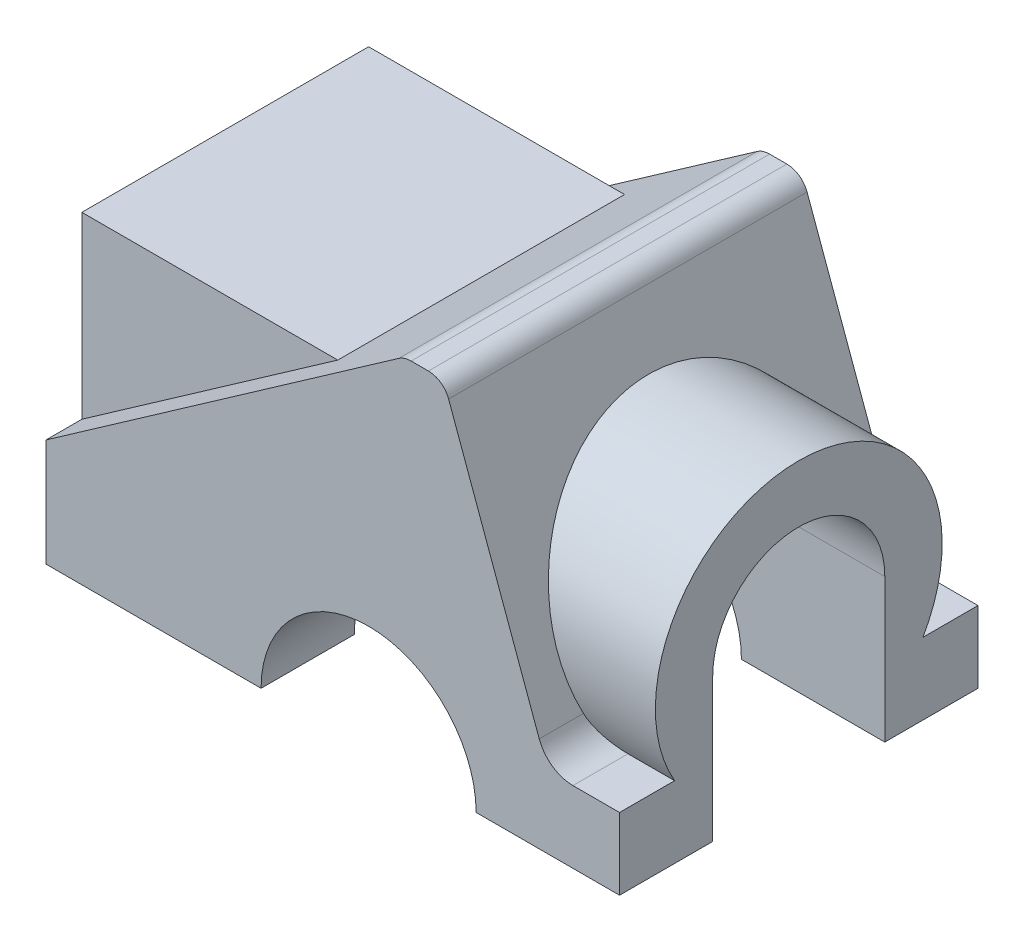
ISO-10303-21;
HEADER;
FILE_DESCRIPTION(('STEP AP214'),'2;1');
FILE_NAME('part.step','',(''),(''),'','','');
FILE_SCHEMA(('AUTOMOTIVE_DESIGN { 1 0 10303 214 1 1 1 1 }'));
ENDSEC;
DATA;
#1=APPLICATION_CONTEXT('core data for automotive mechanical design processes');
#2=APPLICATION_PROTOCOL_DEFINITION('international standard','automotive_design',2000,#1);
#3=PRODUCT_CONTEXT('',#1,'mechanical');
#4=PRODUCT('Part','Part','',(#3));
#5=PRODUCT_RELATED_PRODUCT_CATEGORY('part','',(#4));
#6=PRODUCT_DEFINITION_FORMATION('','',#4);
#7=PRODUCT_DEFINITION_CONTEXT('part definition',#1,'design');
#8=PRODUCT_DEFINITION('design','',#6,#7);
#9=PRODUCT_DEFINITION_SHAPE('','',#8);
#10=(LENGTH_UNIT() NAMED_UNIT(*) SI_UNIT(.MILLI.,.METRE.));
#11=(NAMED_UNIT(*) PLANE_ANGLE_UNIT() SI_UNIT($,.RADIAN.));
#12=(NAMED_UNIT(*) SI_UNIT($,.STERADIAN.) SOLID_ANGLE_UNIT());
#13=UNCERTAINTY_MEASURE_WITH_UNIT(LENGTH_MEASURE(1.E-05),#10,'distance_accuracy_value','');
#14=(GEOMETRIC_REPRESENTATION_CONTEXT(3) GLOBAL_UNCERTAINTY_ASSIGNED_CONTEXT((#13)) GLOBAL_UNIT_ASSIGNED_CONTEXT((#10,
#11,#12)) REPRESENTATION_CONTEXT('',''));
#15=CARTESIAN_POINT('',(0.,0.,0.));
#16=DIRECTION('',(0.,0.,1.));
#17=DIRECTION('',(1.,0.,0.));
#18=AXIS2_PLACEMENT_3D('',#15,#16,#17);
#19=CARTESIAN_POINT('',(-25.,-20.,-25.));
#20=DIRECTION('',(0.,-1.,0.));
#21=DIRECTION('',(0.,0.,-1.));
#22=AXIS2_PLACEMENT_3D('',#19,#20,#21);
#23=PLANE('',#22);
#24=DIRECTION('',(0.,0.,1.));
#25=VECTOR('',#24,1.);
#26=CARTESIAN_POINT('',(-20.,-20.,-25.));
#27=LINE('',#26,#25);
#28=CARTESIAN_POINT('',(-20.,-20.,-25.));
#29=VERTEX_POINT('',#28);
#30=CARTESIAN_POINT('',(-20.,-20.,-12.));
#31=VERTEX_POINT('',#30);
#32=EDGE_CURVE('E201',#29,#31,#27,.T.);
#33=ORIENTED_EDGE('',*,*,#32,.F.);
#34=DIRECTION('',(1.,0.,0.));
#35=VECTOR('',#34,1.);
#36=CARTESIAN_POINT('',(-25.,-20.,-25.));
#37=LINE('',#36,#35);
#38=CARTESIAN_POINT('',(0.,-20.,-25.));
#39=VERTEX_POINT('',#38);
#40=EDGE_CURVE('E213',#29,#39,#37,.T.);
#41=ORIENTED_EDGE('',*,*,#40,.T.);
#42=DIRECTION('',(0.,0.,-1.));
#43=VECTOR('',#42,1.);
#44=CARTESIAN_POINT('',(0.,-20.,-25.));
#45=LINE('',#44,#43);
#46=CARTESIAN_POINT('',(0.,-20.,-12.));
#47=VERTEX_POINT('',#46);
#48=EDGE_CURVE('E435',#47,#39,#45,.T.);
#49=ORIENTED_EDGE('',*,*,#48,.F.);
#50=DIRECTION('',(1.,0.,0.));
#51=VECTOR('',#50,1.);
#52=CARTESIAN_POINT('',(-80.,-20.,-12.));
#53=LINE('',#52,#51);
#54=EDGE_CURVE('E216',#31,#47,#53,.T.);
#55=ORIENTED_EDGE('',*,*,#54,.F.);
#56=EDGE_LOOP('',(#33,#41,#49,#55));
#57=FACE_BOUND('',#56,.T.);
#58=ADVANCED_FACE('F39',(#57),#23,.T.);
#59=CARTESIAN_POINT('',(-20.,-20.,12.));
#60=VERTEX_POINT('',#59);
#61=CARTESIAN_POINT('',(-20.,-20.,25.));
#62=VERTEX_POINT('',#61);
#63=EDGE_CURVE('E218',#60,#62,#27,.T.);
#64=ORIENTED_EDGE('',*,*,#63,.F.);
#65=DIRECTION('',(1.,0.,0.));
#66=VECTOR('',#65,1.);
#67=CARTESIAN_POINT('',(-80.,-20.,12.));
#68=LINE('',#67,#66);
#69=CARTESIAN_POINT('',(0.,-20.,12.));
#70=VERTEX_POINT('',#69);
#71=EDGE_CURVE('E370',#60,#70,#68,.T.);
#72=ORIENTED_EDGE('',*,*,#71,.T.);
#73=CARTESIAN_POINT('',(0.,-20.,25.));
#74=VERTEX_POINT('',#73);
#75=EDGE_CURVE('E433',#74,#70,#45,.T.);
#76=ORIENTED_EDGE('',*,*,#75,.F.);
#77=DIRECTION('',(1.,0.,0.));
#78=VECTOR('',#77,1.);
#79=CARTESIAN_POINT('',(-25.,-20.,25.));
#80=LINE('',#79,#78);
#81=EDGE_CURVE('E238',#62,#74,#80,.T.);
#82=ORIENTED_EDGE('',*,*,#81,.F.);
#83=EDGE_LOOP('',(#64,#72,#76,#82));
#84=FACE_BOUND('',#83,.T.);
#85=ADVANCED_FACE('F320',(#84),#23,.T.);
#86=DIRECTION('',(0.,0.,1.));
#87=VECTOR('',#86,1.);
#88=CARTESIAN_POINT('',(-50.,-20.,-25.));
#89=LINE('',#88,#87);
#90=CARTESIAN_POINT('',(-50.,-20.,-25.));
#91=VERTEX_POINT('',#90);
#92=CARTESIAN_POINT('',(-50.,-20.,-12.));
#93=VERTEX_POINT('',#92);
#94=EDGE_CURVE('E202',#91,#93,#89,.T.);
#95=ORIENTED_EDGE('',*,*,#94,.T.);
#96=CARTESIAN_POINT('',(-80.,-20.,-12.));
#97=VERTEX_POINT('',#96);
#98=EDGE_CURVE('E350',#97,#93,#53,.T.);
#99=ORIENTED_EDGE('',*,*,#98,.F.);
#100=DIRECTION('',(0.,0.,1.));
#101=VECTOR('',#100,1.);
#102=CARTESIAN_POINT('',(-80.,-20.,-20.));
#103=LINE('',#102,#101);
#104=CARTESIAN_POINT('',(-80.,-20.,-25.));
#105=VERTEX_POINT('',#104);
#106=EDGE_CURVE('E401',#105,#97,#103,.T.);
#107=ORIENTED_EDGE('',*,*,#106,.F.);
#108=EDGE_CURVE('E222',#105,#91,#37,.T.);
#109=ORIENTED_EDGE('',*,*,#108,.T.);
#110=EDGE_LOOP('',(#95,#99,#107,#109));
#111=FACE_BOUND('',#110,.T.);
#112=ADVANCED_FACE('F293',(#111),#23,.T.);
#113=CARTESIAN_POINT('',(-25.,0.,0.));
#114=DIRECTION('',(1.,0.,0.));
#115=DIRECTION('',(0.,0.,-1.));
#116=AXIS2_PLACEMENT_3D('',#113,#114,#115);
#117=CYLINDRICAL_SURFACE('',#116,20.);
#118=DIRECTION('',(1.,0.,0.));
#119=VECTOR('',#118,1.);
#120=CARTESIAN_POINT('',(-25.,-10.,-17.3205080756888));
#121=LINE('',#120,#119);
#122=CARTESIAN_POINT('',(-6.50015293830348,-10.,-17.3205080756888));
#123=VERTEX_POINT('',#122);
#124=CARTESIAN_POINT('',(0.,-10.,-17.3205080756888));
#125=VERTEX_POINT('',#124);
#126=EDGE_CURVE('E250',#123,#125,#121,.T.);
#127=ORIENTED_EDGE('',*,*,#126,.F.);
#128=CARTESIAN_POINT('',(-6.50015293830348,-10.,-17.3205080756888));
#129=CARTESIAN_POINT('',(-6.62932598009299,-10.0000238714886,-17.3204823485526));
#130=CARTESIAN_POINT('',(-6.7584853531534,-9.99499539836722,-17.3233971845787));
#131=CARTESIAN_POINT('',(-7.0157192782596,-9.97501366794615,-17.3349169398116));
#132=CARTESIAN_POINT('',(-7.14379431447099,-9.96006510559557,-17.3435191673004));
#133=CARTESIAN_POINT('',(-7.39726993199471,-9.92052515486874,-17.3661643697582));
#134=CARTESIAN_POINT('',(-7.52268090934499,-9.89598396442166,-17.3801790171997));
#135=CARTESIAN_POINT('',(-7.7706253134677,-9.83757393659179,-17.4133073357503));
#136=CARTESIAN_POINT('',(-7.89315851610428,-9.80370437526511,-17.4324214026049));
#137=CARTESIAN_POINT('',(-8.13433492817295,-9.7270949349517,-17.4752837400969));
#138=CARTESIAN_POINT('',(-8.25298474940127,-9.68437115004697,-17.4990235979427));
#139=CARTESIAN_POINT('',(-8.48596795083288,-9.59046145993499,-17.5506672403394));
#140=CARTESIAN_POINT('',(-8.60029966701367,-9.53927233258634,-17.578572610003));
#141=CARTESIAN_POINT('',(-8.93608168037184,-9.37361333523272,-17.667798747046));
#142=CARTESIAN_POINT('',(-9.15025989765532,-9.24707081413842,-17.7346186799669));
#143=CARTESIAN_POINT('',(-9.5692426097082,-8.9560441708774,-17.8834485829157));
#144=CARTESIAN_POINT('',(-9.77236591294091,-8.789536847279,-17.9661907758227));
#145=CARTESIAN_POINT('',(-10.1488054965333,-8.42860836361496,-18.1383169136115));
#146=CARTESIAN_POINT('',(-10.3221135596231,-8.23417953520774,-18.2277026798152));
#147=CARTESIAN_POINT('',(-10.6312683867996,-7.8278869436768,-18.4057530078534));
#148=CARTESIAN_POINT('',(-10.768118765279,-7.61676033549982,-18.4943524146803));
#149=CARTESIAN_POINT('',(-10.9485551203868,-7.28636689423075,-18.6258678959415));
#150=CARTESIAN_POINT('',(-11.0045475999084,-7.17398766653187,-18.669462887011));
#151=CARTESIAN_POINT('',(-11.1080265971445,-6.94506150217783,-18.7558287027057));
#152=CARTESIAN_POINT('',(-11.1555124013709,-6.82851421691391,-18.7985994579308));
#153=CARTESIAN_POINT('',(-11.198616042233,-6.71010071662832,-18.8407682532508));
#154=B_SPLINE_CURVE_WITH_KNOTS('',3,(#128,#129,#130,#131,#132,#133,#134,#135,#136,#137,#138,
#139,#140,#141,#142,#143,#144,#145,#146,#147,#148,#149,#150,#151,#152,#153),.UNSPECIFIED.,.F.,
.F.,(4,2,2,2,2,2,2,2,2,2,2,2,4),(0.,0.387366916483921,0.774550631777033,1.15973478240918,
1.54494883433132,1.92946873960573,2.31413534198989,3.08365501065917,3.90656154736029,
4.72969452026274,5.52703670416455,5.92546831404102,6.32393332630645),.UNSPECIFIED.);
#155=CARTESIAN_POINT('',(-11.198616042233,-6.71010071662833,-18.8407682532508));
#156=VERTEX_POINT('',#155);
#157=EDGE_CURVE('E276',#123,#156,#154,.T.);
#158=ORIENTED_EDGE('',*,*,#157,.T.);
#159=CARTESIAN_POINT('',(-13.640892972014,0.,0.));
#160=DIRECTION('',(-0.939692620785909,-0.342020143325666,0.));
#161=DIRECTION('',(0.342020143325666,-0.93969262078591,0.));
#162=AXIS2_PLACEMENT_3D('',#159,#160,#161);
#163=ELLIPSE('',#162,21.2835554495182,20.);
#164=CARTESIAN_POINT('',(-11.198616042233,-6.71010071662832,18.8407682532508));
#165=VERTEX_POINT('',#164);
#166=EDGE_CURVE('E396',#156,#165,#163,.F.);
#167=ORIENTED_EDGE('',*,*,#166,.T.);
#168=CARTESIAN_POINT('',(-11.198616042233,-6.71010071662832,18.8407682532508));
#169=CARTESIAN_POINT('',(-11.1478933001544,-6.84946739754972,18.7911457978657));
#170=CARTESIAN_POINT('',(-11.091070283619,-6.98628702590569,18.7406628073047));
#171=CARTESIAN_POINT('',(-10.9657074940171,-7.25403332861618,18.6386533477071));
#172=CARTESIAN_POINT('',(-10.8971684601529,-7.38496037409518,18.5871269446834));
#173=CARTESIAN_POINT('',(-10.7486815567545,-7.64043181151173,18.4835837294399));
#174=CARTESIAN_POINT('',(-10.668707990932,-7.76496094495089,18.4315660660118));
#175=CARTESIAN_POINT('',(-10.4979879965461,-8.00652695314276,18.3279248102382));
#176=CARTESIAN_POINT('',(-10.4072414075635,-8.12356371628792,18.2763012237731));
#177=CARTESIAN_POINT('',(-10.1194992441027,-8.46238060412113,18.1231710992993));
#178=CARTESIAN_POINT('',(-9.90691703329392,-8.6720121680441,18.0233454361635));
#179=CARTESIAN_POINT('',(-9.4446192931982,-9.05209761344705,17.8354879565025));
#180=CARTESIAN_POINT('',(-9.19492201551797,-9.22257064712734,17.7474503833196));
#181=CARTESIAN_POINT('',(-8.80207214209825,-9.44101267056508,17.6316125587938));
#182=CARTESIAN_POINT('',(-8.67074314265878,-9.5066917802394,17.5962348123772));
#183=CARTESIAN_POINT('',(-8.40170858795586,-9.62663336357725,17.5309038264555));
#184=CARTESIAN_POINT('',(-8.26400658596734,-9.68090210772967,17.500947608853));
#185=CARTESIAN_POINT('',(-7.98349929240674,-9.77719982667535,17.4473323071006));
#186=CARTESIAN_POINT('',(-7.84070412904771,-9.81925172175522,17.4236614381505));
#187=CARTESIAN_POINT('',(-7.55106963492899,-9.89058253846352,17.3832693868561));
#188=CARTESIAN_POINT('',(-7.40423289511326,-9.91986944954611,17.3665438578158));
#189=CARTESIAN_POINT('',(-7.13131252847476,-9.96160834532938,17.342631432531));
#190=CARTESIAN_POINT('',(-7.00561575565265,-9.97598919304104,17.3343549330109));
#191=CARTESIAN_POINT('',(-6.75333769753141,-9.9951919703866,17.3232838074443));
#192=CARTESIAN_POINT('',(-6.62675703152767,-10.0000200275496,17.3204856673784));
#193=CARTESIAN_POINT('',(-6.50015293830348,-9.99999999999999,17.3205080756888));
#194=B_SPLINE_CURVE_WITH_KNOTS('',3,(#168,#169,#170,#171,#172,#173,#174,#175,#176,#177,#178,
#179,#180,#181,#182,#183,#184,#185,#186,#187,#188,#189,#190,#191,#192,#193),.UNSPECIFIED.,.F.,
.F.,(4,2,2,2,2,2,2,2,2,2,2,2,4),(0.,0.469004212934333,0.937978845763651,1.4080244497972,
1.87807705407625,2.8176553016317,3.75677302400749,4.20934155211913,4.66166072045004,
5.11312572056472,5.56430774682961,5.94419925761307,6.3238470121974),.UNSPECIFIED.);
#195=CARTESIAN_POINT('',(-6.50015293830348,-10.,17.3205080756888));
#196=VERTEX_POINT('',#195);
#197=EDGE_CURVE('E64',#165,#196,#194,.T.);
#198=ORIENTED_EDGE('',*,*,#197,.T.);
#199=DIRECTION('',(1.,0.,0.));
#200=VECTOR('',#199,1.);
#201=CARTESIAN_POINT('',(-25.,-10.,17.3205080756888));
#202=LINE('',#201,#200);
#203=CARTESIAN_POINT('',(0.,-10.,17.3205080756888));
#204=VERTEX_POINT('',#203);
#205=EDGE_CURVE('E241',#196,#204,#202,.T.);
#206=ORIENTED_EDGE('',*,*,#205,.T.);
#207=CARTESIAN_POINT('',(0.,0.,0.));
#208=DIRECTION('',(1.,0.,0.));
#209=DIRECTION('',(0.,0.,1.));
#210=AXIS2_PLACEMENT_3D('',#207,#208,#209);
#211=CIRCLE('',#210,20.);
#212=EDGE_CURVE('E413',#125,#204,#211,.T.);
#213=ORIENTED_EDGE('',*,*,#212,.F.);
#214=EDGE_LOOP('',(#127,#158,#167,#198,#206,#213));
#215=FACE_BOUND('',#214,.T.);
#216=ADVANCED_FACE('F282',(#215),#117,.T.);
#217=CARTESIAN_POINT('',(-25.,-10.,-17.3205080756888));
#218=DIRECTION('',(0.,1.,0.));
#219=DIRECTION('',(0.,0.,1.));
#220=AXIS2_PLACEMENT_3D('',#217,#218,#219);
#221=PLANE('',#220);
#222=DIRECTION('',(1.,0.,0.));
#223=VECTOR('',#222,1.);
#224=CARTESIAN_POINT('',(-25.,-10.,-25.));
#225=LINE('',#224,#223);
#226=CARTESIAN_POINT('',(-6.50015293830348,-10.,-25.));
#227=VERTEX_POINT('',#226);
#228=CARTESIAN_POINT('',(0.,-10.,-25.));
#229=VERTEX_POINT('',#228);
#230=EDGE_CURVE('E226',#227,#229,#225,.T.);
#231=ORIENTED_EDGE('',*,*,#230,.F.);
#232=DIRECTION('',(0.,0.,-1.));
#233=VECTOR('',#232,1.);
#234=CARTESIAN_POINT('',(-6.50015293830348,-10.,-17.3205080756888));
#235=LINE('',#234,#233);
#236=EDGE_CURVE('E272',#227,#123,#235,.F.);
#237=ORIENTED_EDGE('',*,*,#236,.T.);
#238=ORIENTED_EDGE('',*,*,#126,.T.);
#239=DIRECTION('',(0.,0.,1.));
#240=VECTOR('',#239,1.);
#241=CARTESIAN_POINT('',(0.,-10.,-17.3205080756888));
#242=LINE('',#241,#240);
#243=EDGE_CURVE('E243',#229,#125,#242,.T.);
#244=ORIENTED_EDGE('',*,*,#243,.F.);
#245=EDGE_LOOP('',(#231,#237,#238,#244));
#246=FACE_BOUND('',#245,.T.);
#247=ADVANCED_FACE('F287',(#246),#221,.T.);
#248=CARTESIAN_POINT('',(-25.,0.,-12.));
#249=DIRECTION('',(0.,0.,1.));
#250=DIRECTION('',(1.,0.,0.));
#251=AXIS2_PLACEMENT_3D('',#248,#249,#250);
#252=PLANE('',#251);
#253=CARTESIAN_POINT('',(-35.,-20.,-12.));
#254=DIRECTION('',(0.,0.,1.));
#255=DIRECTION('',(1.,0.,0.));
#256=AXIS2_PLACEMENT_3D('',#253,#254,#255);
#257=CIRCLE('',#256,15.);
#258=EDGE_CURVE('E355',#31,#93,#257,.T.);
#259=ORIENTED_EDGE('',*,*,#258,.F.);
#260=ORIENTED_EDGE('',*,*,#54,.T.);
#261=DIRECTION('',(0.,-1.,0.));
#262=VECTOR('',#261,1.);
#263=CARTESIAN_POINT('',(0.,0.,-12.));
#264=LINE('',#263,#262);
#265=CARTESIAN_POINT('',(0.,0.,-12.));
#266=VERTEX_POINT('',#265);
#267=EDGE_CURVE('E429',#266,#47,#264,.T.);
#268=ORIENTED_EDGE('',*,*,#267,.F.);
#269=DIRECTION('',(1.,0.,0.));
#270=VECTOR('',#269,1.);
#271=CARTESIAN_POINT('',(-25.,0.,-12.));
#272=LINE('',#271,#270);
#273=CARTESIAN_POINT('',(-80.,0.,-12.));
#274=VERTEX_POINT('',#273);
#275=EDGE_CURVE('E228',#274,#266,#272,.T.);
#276=ORIENTED_EDGE('',*,*,#275,.F.);
#277=DIRECTION('',(0.,1.,0.));
#278=VECTOR('',#277,1.);
#279=CARTESIAN_POINT('',(-80.,-20.,-12.));
#280=LINE('',#279,#278);
#281=EDGE_CURVE('E352',#97,#274,#280,.T.);
#282=ORIENTED_EDGE('',*,*,#281,.F.);
#283=ORIENTED_EDGE('',*,*,#98,.T.);
#284=EDGE_LOOP('',(#259,#260,#268,#276,#282,#283));
#285=FACE_BOUND('',#284,.T.);
#286=ADVANCED_FACE('F351',(#285),#252,.T.);
#287=CARTESIAN_POINT('',(-25.,0.,0.));
#288=DIRECTION('',(1.,0.,0.));
#289=DIRECTION('',(0.,0.,-1.));
#290=AXIS2_PLACEMENT_3D('',#287,#288,#289);
#291=CYLINDRICAL_SURFACE('',#290,12.);
#292=DIRECTION('',(1.,0.,0.));
#293=VECTOR('',#292,1.);
#294=CARTESIAN_POINT('',(-25.,0.,12.));
#295=LINE('',#294,#293);
#296=CARTESIAN_POINT('',(-80.,0.,12.));
#297=VERTEX_POINT('',#296);
#298=CARTESIAN_POINT('',(0.,0.,12.));
#299=VERTEX_POINT('',#298);
#300=EDGE_CURVE('E230',#297,#299,#295,.T.);
#301=ORIENTED_EDGE('',*,*,#300,.F.);
#302=CARTESIAN_POINT('',(-80.,0.,0.));
#303=DIRECTION('',(1.,0.,0.));
#304=DIRECTION('',(0.,0.,-1.));
#305=AXIS2_PLACEMENT_3D('',#302,#303,#304);
#306=CIRCLE('',#305,12.);
#307=EDGE_CURVE('E494',#274,#297,#306,.T.);
#308=ORIENTED_EDGE('',*,*,#307,.F.);
#309=ORIENTED_EDGE('',*,*,#275,.T.);
#310=CARTESIAN_POINT('',(0.,0.,0.));
#311=DIRECTION('',(-1.,0.,0.));
#312=DIRECTION('',(0.,0.,1.));
#313=AXIS2_PLACEMENT_3D('',#310,#311,#312);
#314=CIRCLE('',#313,12.);
#315=EDGE_CURVE('E428',#299,#266,#314,.T.);
#316=ORIENTED_EDGE('',*,*,#315,.F.);
#317=EDGE_LOOP('',(#301,#308,#309,#316));
#318=FACE_BOUND('',#317,.T.);
#319=ADVANCED_FACE('F452',(#318),#291,.F.);
#320=CARTESIAN_POINT('',(-25.,0.,12.));
#321=DIRECTION('',(0.,0.,-1.));
#322=DIRECTION('',(0.,1.,0.));
#323=AXIS2_PLACEMENT_3D('',#320,#321,#322);
#324=PLANE('',#323);
#325=CARTESIAN_POINT('',(-35.,-20.,12.));
#326=DIRECTION('',(0.,0.,-1.));
#327=DIRECTION('',(0.,1.,0.));
#328=AXIS2_PLACEMENT_3D('',#325,#326,#327);
#329=CIRCLE('',#328,15.);
#330=CARTESIAN_POINT('',(-50.,-20.,12.));
#331=VERTEX_POINT('',#330);
#332=EDGE_CURVE('E220',#331,#60,#329,.T.);
#333=ORIENTED_EDGE('',*,*,#332,.F.);
#334=CARTESIAN_POINT('',(-80.,-20.,12.));
#335=VERTEX_POINT('',#334);
#336=EDGE_CURVE('E363',#335,#331,#68,.T.);
#337=ORIENTED_EDGE('',*,*,#336,.F.);
#338=DIRECTION('',(0.,-1.,0.));
#339=VECTOR('',#338,1.);
#340=CARTESIAN_POINT('',(-80.,-10.,12.));
#341=LINE('',#340,#339);
#342=EDGE_CURVE('E493',#297,#335,#341,.T.);
#343=ORIENTED_EDGE('',*,*,#342,.F.);
#344=ORIENTED_EDGE('',*,*,#300,.T.);
#345=DIRECTION('',(0.,1.,0.));
#346=VECTOR('',#345,1.);
#347=CARTESIAN_POINT('',(0.,0.,12.));
#348=LINE('',#347,#346);
#349=EDGE_CURVE('E421',#70,#299,#348,.T.);
#350=ORIENTED_EDGE('',*,*,#349,.F.);
#351=ORIENTED_EDGE('',*,*,#71,.F.);
#352=EDGE_LOOP('',(#333,#337,#343,#344,#350,#351));
#353=FACE_BOUND('',#352,.T.);
#354=ADVANCED_FACE('F489',(#353),#324,.T.);
#355=CARTESIAN_POINT('',(-25.,-10.,17.3205080756888));
#356=DIRECTION('',(0.,1.,0.));
#357=DIRECTION('',(0.,0.,1.));
#358=AXIS2_PLACEMENT_3D('',#355,#356,#357);
#359=PLANE('',#358);
#360=ORIENTED_EDGE('',*,*,#205,.F.);
#361=DIRECTION('',(0.,0.,-1.));
#362=VECTOR('',#361,1.);
#363=CARTESIAN_POINT('',(-6.50015293830348,-10.,17.3205080756888));
#364=LINE('',#363,#362);
#365=CARTESIAN_POINT('',(-6.50015293830348,-10.,25.));
#366=VERTEX_POINT('',#365);
#367=EDGE_CURVE('E54',#196,#366,#364,.F.);
#368=ORIENTED_EDGE('',*,*,#367,.T.);
#369=DIRECTION('',(1.,0.,0.));
#370=VECTOR('',#369,1.);
#371=CARTESIAN_POINT('',(-25.,-10.,25.));
#372=LINE('',#371,#370);
#373=CARTESIAN_POINT('',(0.,-10.,25.));
#374=VERTEX_POINT('',#373);
#375=EDGE_CURVE('E237',#366,#374,#372,.T.);
#376=ORIENTED_EDGE('',*,*,#375,.T.);
#377=DIRECTION('',(0.,0.,1.));
#378=VECTOR('',#377,1.);
#379=CARTESIAN_POINT('',(0.,-10.,17.3205080756888));
#380=LINE('',#379,#378);
#381=EDGE_CURVE('E416',#204,#374,#380,.T.);
#382=ORIENTED_EDGE('',*,*,#381,.F.);
#383=EDGE_LOOP('',(#360,#368,#376,#382));
#384=FACE_BOUND('',#383,.T.);
#385=ADVANCED_FACE('F292',(#384),#359,.T.);
#386=CARTESIAN_POINT('',(-80.,-20.,-20.));
#387=DIRECTION('',(0.,0.,1.));
#388=DIRECTION('',(1.,0.,0.));
#389=AXIS2_PLACEMENT_3D('',#386,#387,#388);
#390=PLANE('',#389);
#391=DIRECTION('',(0.819152044288991,0.573576436351047,0.));
#392=VECTOR('',#391,1.);
#393=CARTESIAN_POINT('',(-87.0489119740813,-9.93311041451516,-20.));
#394=LINE('',#393,#392);
#395=CARTESIAN_POINT('',(-80.,-4.99740911408671,-20.));
#396=VERTEX_POINT('',#395);
#397=CARTESIAN_POINT('',(-44.3,20.,-20.));
#398=VERTEX_POINT('',#397);
#399=EDGE_CURVE('E393',#396,#398,#394,.T.);
#400=ORIENTED_EDGE('',*,*,#399,.F.);
#401=DIRECTION('',(0.,-1.,0.));
#402=VECTOR('',#401,1.);
#403=CARTESIAN_POINT('',(-80.,-20.,-20.));
#404=LINE('',#403,#402);
#405=CARTESIAN_POINT('',(-80.,20.,-20.));
#406=VERTEX_POINT('',#405);
#407=EDGE_CURVE('E398',#406,#396,#404,.T.);
#408=ORIENTED_EDGE('',*,*,#407,.F.);
#409=DIRECTION('',(1.,0.,0.));
#410=VECTOR('',#409,1.);
#411=CARTESIAN_POINT('',(-80.,20.,-20.));
#412=LINE('',#411,#410);
#413=EDGE_CURVE('E406',#406,#398,#412,.T.);
#414=ORIENTED_EDGE('',*,*,#413,.T.);
#415=EDGE_LOOP('',(#400,#408,#414));
#416=FACE_BOUND('',#415,.T.);
#417=ADVANCED_FACE('F459',(#416),#390,.F.);
#418=CARTESIAN_POINT('',(-80.,-20.,20.));
#419=DIRECTION('',(0.,0.,-1.));
#420=DIRECTION('',(-1.,0.,0.));
#421=AXIS2_PLACEMENT_3D('',#418,#419,#420);
#422=PLANE('',#421);
#423=DIRECTION('',(-0.819152044288991,-0.573576436351047,0.));
#424=VECTOR('',#423,1.);
#425=CARTESIAN_POINT('',(-87.0489119740813,-9.93311041451516,20.));
#426=LINE('',#425,#424);
#427=CARTESIAN_POINT('',(-44.3,20.,20.));
#428=VERTEX_POINT('',#427);
#429=CARTESIAN_POINT('',(-80.,-4.99740911408671,20.));
#430=VERTEX_POINT('',#429);
#431=EDGE_CURVE('E394',#428,#430,#426,.T.);
#432=ORIENTED_EDGE('',*,*,#431,.F.);
#433=DIRECTION('',(1.,0.,0.));
#434=VECTOR('',#433,1.);
#435=CARTESIAN_POINT('',(-80.,20.,20.));
#436=LINE('',#435,#434);
#437=CARTESIAN_POINT('',(-80.,20.,20.));
#438=VERTEX_POINT('',#437);
#439=EDGE_CURVE('E411',#438,#428,#436,.T.);
#440=ORIENTED_EDGE('',*,*,#439,.F.);
#441=DIRECTION('',(0.,1.,0.));
#442=VECTOR('',#441,1.);
#443=CARTESIAN_POINT('',(-80.,-20.,20.));
#444=LINE('',#443,#442);
#445=EDGE_CURVE('E403',#430,#438,#444,.T.);
#446=ORIENTED_EDGE('',*,*,#445,.F.);
#447=EDGE_LOOP('',(#432,#440,#446));
#448=FACE_BOUND('',#447,.T.);
#449=ADVANCED_FACE('F458',(#448),#422,.F.);
#450=CARTESIAN_POINT('',(-80.,20.,-20.));
#451=DIRECTION('',(0.,-1.,0.));
#452=DIRECTION('',(0.,0.,-1.));
#453=AXIS2_PLACEMENT_3D('',#450,#451,#452);
#454=PLANE('',#453);
#455=DIRECTION('',(0.,0.,1.));
#456=VECTOR('',#455,1.);
#457=CARTESIAN_POINT('',(-44.3,20.,-20.));
#458=LINE('',#457,#456);
#459=EDGE_CURVE('E389',#398,#428,#458,.T.);
#460=ORIENTED_EDGE('',*,*,#459,.F.);
#461=ORIENTED_EDGE('',*,*,#413,.F.);
#462=DIRECTION('',(0.,0.,-1.));
#463=VECTOR('',#462,1.);
#464=CARTESIAN_POINT('',(-80.,20.,-20.));
#465=LINE('',#464,#463);
#466=EDGE_CURVE('E410',#438,#406,#465,.T.);
#467=ORIENTED_EDGE('',*,*,#466,.F.);
#468=ORIENTED_EDGE('',*,*,#439,.T.);
#469=EDGE_LOOP('',(#460,#461,#467,#468));
#470=FACE_BOUND('',#469,.T.);
#471=ADVANCED_FACE('F336',(#470),#454,.F.);
#472=CARTESIAN_POINT('',(-25.,-10.,-25.));
#473=DIRECTION('',(0.,0.,-1.));
#474=DIRECTION('',(-1.,0.,0.));
#475=AXIS2_PLACEMENT_3D('',#472,#473,#474);
#476=PLANE('',#475);
#477=CARTESIAN_POINT('',(-35.,-20.,-25.));
#478=DIRECTION('',(0.,0.,1.));
#479=DIRECTION('',(-1.,0.,0.));
#480=AXIS2_PLACEMENT_3D('',#477,#478,#479);
#481=CIRCLE('',#480,15.);
#482=EDGE_CURVE('E198',#29,#91,#481,.T.);
#483=ORIENTED_EDGE('',*,*,#482,.T.);
#484=ORIENTED_EDGE('',*,*,#108,.F.);
#485=DIRECTION('',(0.,-1.,0.));
#486=VECTOR('',#485,1.);
#487=CARTESIAN_POINT('',(-80.,-4.99740911408671,-25.));
#488=LINE('',#487,#486);
#489=CARTESIAN_POINT('',(-80.,-4.99740911408671,-25.));
#490=VERTEX_POINT('',#489);
#491=EDGE_CURVE('E358',#490,#105,#488,.T.);
#492=ORIENTED_EDGE('',*,*,#491,.F.);
#493=DIRECTION('',(-0.819152044288991,-0.573576436351047,0.));
#494=VECTOR('',#493,1.);
#495=CARTESIAN_POINT('',(-80.,-4.99740911408671,-25.));
#496=LINE('',#495,#494);
#497=CARTESIAN_POINT('',(-30.7933528749951,29.457456132867,-25.));
#498=VERTEX_POINT('',#497);
#499=EDGE_CURVE('E375',#498,#490,#496,.T.);
#500=ORIENTED_EDGE('',*,*,#499,.F.);
#501=CARTESIAN_POINT('',(-29.0726235659419,27.,-25.));
#502=DIRECTION('',(0.,0.,-1.));
#503=DIRECTION('',(-1.,0.,0.));
#504=AXIS2_PLACEMENT_3D('',#501,#502,#503);
#505=CIRCLE('',#504,3.);
#506=CARTESIAN_POINT('',(-29.0726235659419,30.,-25.));
#507=VERTEX_POINT('',#506);
#508=EDGE_CURVE('E249',#498,#507,#505,.T.);
#509=ORIENTED_EDGE('',*,*,#508,.T.);
#510=DIRECTION('',(-1.,0.,0.));
#511=VECTOR('',#510,1.);
#512=CARTESIAN_POINT('',(-30.0185199325789,30.,-25.));
#513=LINE('',#512,#511);
#514=CARTESIAN_POINT('',(-26.6606226146291,30.,-25.));
#515=VERTEX_POINT('',#514);
#516=EDGE_CURVE('E382',#515,#507,#513,.T.);
#517=ORIENTED_EDGE('',*,*,#516,.F.);
#518=CARTESIAN_POINT('',(-26.6606226146291,27.,-25.));
#519=DIRECTION('',(0.,0.,-1.));
#520=DIRECTION('',(-1.,0.,0.));
#521=AXIS2_PLACEMENT_3D('',#518,#519,#520);
#522=CIRCLE('',#521,3.);
#523=CARTESIAN_POINT('',(-23.8415447522714,28.026060429977,-25.));
#524=VERTEX_POINT('',#523);
#525=EDGE_CURVE('E255',#515,#524,#522,.T.);
#526=ORIENTED_EDGE('',*,*,#525,.T.);
#527=DIRECTION('',(-0.342020143325666,0.939692620785909,0.));
#528=VECTOR('',#527,1.);
#529=CARTESIAN_POINT('',(-24.56,30.,-25.));
#530=LINE('',#529,#528);
#531=CARTESIAN_POINT('',(-11.198616042233,-6.71010071662833,-25.));
#532=VERTEX_POINT('',#531);
#533=EDGE_CURVE('E360',#532,#524,#530,.T.);
#534=ORIENTED_EDGE('',*,*,#533,.F.);
#535=CARTESIAN_POINT('',(-6.50015293830348,-4.99999999999999,-25.));
#536=DIRECTION('',(0.,0.,-1.));
#537=DIRECTION('',(-1.,0.,0.));
#538=AXIS2_PLACEMENT_3D('',#535,#536,#537);
#539=CIRCLE('',#538,5.);
#540=EDGE_CURVE('E48',#532,#227,#539,.F.);
#541=ORIENTED_EDGE('',*,*,#540,.T.);
#542=ORIENTED_EDGE('',*,*,#230,.T.);
#543=DIRECTION('',(0.,1.,0.));
#544=VECTOR('',#543,1.);
#545=CARTESIAN_POINT('',(0.,-10.,-25.));
#546=LINE('',#545,#544);
#547=EDGE_CURVE('E223',#39,#229,#546,.T.);
#548=ORIENTED_EDGE('',*,*,#547,.F.);
#549=ORIENTED_EDGE('',*,*,#40,.F.);
#550=EDGE_LOOP('',(#483,#484,#492,#500,#509,#517,#526,#534,#541,#542,#548,#549));
#551=FACE_BOUND('',#550,.T.);
#552=ADVANCED_FACE('F221',(#551),#476,.T.);
#553=CARTESIAN_POINT('',(-50.,-20.,25.));
#554=VERTEX_POINT('',#553);
#555=EDGE_CURVE('E209',#331,#554,#89,.T.);
#556=ORIENTED_EDGE('',*,*,#555,.T.);
#557=CARTESIAN_POINT('',(-80.,-20.,25.));
#558=VERTEX_POINT('',#557);
#559=EDGE_CURVE('E232',#558,#554,#80,.T.);
#560=ORIENTED_EDGE('',*,*,#559,.F.);
#561=EDGE_CURVE('E405',#335,#558,#103,.T.);
#562=ORIENTED_EDGE('',*,*,#561,.F.);
#563=ORIENTED_EDGE('',*,*,#336,.T.);
#564=EDGE_LOOP('',(#556,#560,#562,#563));
#565=FACE_BOUND('',#564,.T.);
#566=ADVANCED_FACE('F316',(#565),#23,.T.);
#567=CARTESIAN_POINT('',(-25.,-10.,25.));
#568=DIRECTION('',(0.,0.,1.));
#569=DIRECTION('',(1.,0.,0.));
#570=AXIS2_PLACEMENT_3D('',#567,#568,#569);
#571=PLANE('',#570);
#572=CARTESIAN_POINT('',(-35.,-20.,25.));
#573=DIRECTION('',(0.,0.,1.));
#574=DIRECTION('',(-1.,0.,0.));
#575=AXIS2_PLACEMENT_3D('',#572,#573,#574);
#576=CIRCLE('',#575,15.);
#577=EDGE_CURVE('E208',#62,#554,#576,.T.);
#578=ORIENTED_EDGE('',*,*,#577,.F.);
#579=ORIENTED_EDGE('',*,*,#81,.T.);
#580=DIRECTION('',(0.,-1.,0.));
#581=VECTOR('',#580,1.);
#582=CARTESIAN_POINT('',(0.,-10.,25.));
#583=LINE('',#582,#581);
#584=EDGE_CURVE('E417',#374,#74,#583,.T.);
#585=ORIENTED_EDGE('',*,*,#584,.F.);
#586=ORIENTED_EDGE('',*,*,#375,.F.);
#587=CARTESIAN_POINT('',(-6.50015293830348,-4.99999999999999,25.));
#588=DIRECTION('',(0.,0.,1.));
#589=DIRECTION('',(1.,0.,0.));
#590=AXIS2_PLACEMENT_3D('',#587,#588,#589);
#591=CIRCLE('',#590,5.);
#592=CARTESIAN_POINT('',(-11.198616042233,-6.71010071662831,25.));
#593=VERTEX_POINT('',#592);
#594=EDGE_CURVE('E11',#366,#593,#591,.F.);
#595=ORIENTED_EDGE('',*,*,#594,.T.);
#596=DIRECTION('',(-0.342020143325666,0.939692620785909,0.));
#597=VECTOR('',#596,1.);
#598=CARTESIAN_POINT('',(-24.56,30.,25.));
#599=LINE('',#598,#597);
#600=CARTESIAN_POINT('',(-23.8415447522714,28.026060429977,25.));
#601=VERTEX_POINT('',#600);
#602=EDGE_CURVE('E371',#593,#601,#599,.T.);
#603=ORIENTED_EDGE('',*,*,#602,.T.);
#604=CARTESIAN_POINT('',(-26.6606226146291,27.,25.));
#605=DIRECTION('',(0.,0.,1.));
#606=DIRECTION('',(1.,0.,0.));
#607=AXIS2_PLACEMENT_3D('',#604,#605,#606);
#608=CIRCLE('',#607,3.);
#609=CARTESIAN_POINT('',(-26.6606226146291,30.,25.));
#610=VERTEX_POINT('',#609);
#611=EDGE_CURVE('E258',#601,#610,#608,.T.);
#612=ORIENTED_EDGE('',*,*,#611,.T.);
#613=DIRECTION('',(-1.,0.,0.));
#614=VECTOR('',#613,1.);
#615=CARTESIAN_POINT('',(-30.0185199325789,30.,25.));
#616=LINE('',#615,#614);
#617=CARTESIAN_POINT('',(-29.0726235659419,30.,25.));
#618=VERTEX_POINT('',#617);
#619=EDGE_CURVE('E372',#610,#618,#616,.T.);
#620=ORIENTED_EDGE('',*,*,#619,.T.);
#621=CARTESIAN_POINT('',(-29.0726235659419,27.,25.));
#622=DIRECTION('',(0.,0.,1.));
#623=DIRECTION('',(1.,0.,0.));
#624=AXIS2_PLACEMENT_3D('',#621,#622,#623);
#625=CIRCLE('',#624,3.);
#626=CARTESIAN_POINT('',(-30.7933528749951,29.457456132867,25.));
#627=VERTEX_POINT('',#626);
#628=EDGE_CURVE('E259',#618,#627,#625,.T.);
#629=ORIENTED_EDGE('',*,*,#628,.T.);
#630=DIRECTION('',(-0.819152044288991,-0.573576436351047,0.));
#631=VECTOR('',#630,1.);
#632=CARTESIAN_POINT('',(-80.,-4.99740911408671,25.));
#633=LINE('',#632,#631);
#634=CARTESIAN_POINT('',(-80.,-4.99740911408671,25.));
#635=VERTEX_POINT('',#634);
#636=EDGE_CURVE('E380',#627,#635,#633,.T.);
#637=ORIENTED_EDGE('',*,*,#636,.T.);
#638=DIRECTION('',(0.,-1.,0.));
#639=VECTOR('',#638,1.);
#640=CARTESIAN_POINT('',(-80.,-4.99740911408671,25.));
#641=LINE('',#640,#639);
#642=EDGE_CURVE('E368',#635,#558,#641,.T.);
#643=ORIENTED_EDGE('',*,*,#642,.T.);
#644=ORIENTED_EDGE('',*,*,#559,.T.);
#645=EDGE_LOOP('',(#578,#579,#585,#586,#595,#603,#612,#620,#629,#637,#643,#644));
#646=FACE_BOUND('',#645,.T.);
#647=ADVANCED_FACE('F330',(#646),#571,.T.);
#648=CARTESIAN_POINT('',(0.,0.,0.));
#649=DIRECTION('',(-1.,0.,0.));
#650=DIRECTION('',(0.,0.,1.));
#651=AXIS2_PLACEMENT_3D('',#648,#649,#650);
#652=PLANE('',#651);
#653=ORIENTED_EDGE('',*,*,#267,.T.);
#654=ORIENTED_EDGE('',*,*,#48,.T.);
#655=ORIENTED_EDGE('',*,*,#547,.T.);
#656=ORIENTED_EDGE('',*,*,#243,.T.);
#657=ORIENTED_EDGE('',*,*,#212,.T.);
#658=ORIENTED_EDGE('',*,*,#381,.T.);
#659=ORIENTED_EDGE('',*,*,#584,.T.);
#660=ORIENTED_EDGE('',*,*,#75,.T.);
#661=ORIENTED_EDGE('',*,*,#349,.T.);
#662=ORIENTED_EDGE('',*,*,#315,.T.);
#663=EDGE_LOOP('',(#653,#654,#655,#656,#657,#658,#659,#660,#661,#662));
#664=FACE_BOUND('',#663,.T.);
#665=ADVANCED_FACE('F332',(#664),#652,.F.);
#666=CARTESIAN_POINT('',(-80.,0.,0.));
#667=DIRECTION('',(1.,0.,0.));
#668=DIRECTION('',(0.,0.,-1.));
#669=AXIS2_PLACEMENT_3D('',#666,#667,#668);
#670=PLANE('',#669);
#671=ORIENTED_EDGE('',*,*,#106,.T.);
#672=ORIENTED_EDGE('',*,*,#281,.T.);
#673=ORIENTED_EDGE('',*,*,#307,.T.);
#674=ORIENTED_EDGE('',*,*,#342,.T.);
#675=ORIENTED_EDGE('',*,*,#561,.T.);
#676=ORIENTED_EDGE('',*,*,#642,.F.);
#677=DIRECTION('',(0.,0.,-1.));
#678=VECTOR('',#677,1.);
#679=CARTESIAN_POINT('',(-80.,-4.99740911408671,25.));
#680=LINE('',#679,#678);
#681=EDGE_CURVE('E383',#635,#430,#680,.T.);
#682=ORIENTED_EDGE('',*,*,#681,.T.);
#683=ORIENTED_EDGE('',*,*,#445,.T.);
#684=ORIENTED_EDGE('',*,*,#466,.T.);
#685=ORIENTED_EDGE('',*,*,#407,.T.);
#686=EDGE_CURVE('E377',#396,#490,#680,.T.);
#687=ORIENTED_EDGE('',*,*,#686,.T.);
#688=ORIENTED_EDGE('',*,*,#491,.T.);
#689=EDGE_LOOP('',(#671,#672,#673,#674,#675,#676,#682,#683,#684,#685,#687,#688));
#690=FACE_BOUND('',#689,.T.);
#691=ADVANCED_FACE('F453',(#690),#670,.F.);
#692=CARTESIAN_POINT('',(-30.0185199325789,30.,25.));
#693=DIRECTION('',(0.,-1.,0.));
#694=DIRECTION('',(0.,0.,-1.));
#695=AXIS2_PLACEMENT_3D('',#692,#693,#694);
#696=PLANE('',#695);
#697=ORIENTED_EDGE('',*,*,#619,.F.);
#698=DIRECTION('',(0.,0.,-1.));
#699=VECTOR('',#698,1.);
#700=CARTESIAN_POINT('',(-26.6606226146291,30.,25.));
#701=LINE('',#700,#699);
#702=EDGE_CURVE('E246',#610,#515,#701,.T.);
#703=ORIENTED_EDGE('',*,*,#702,.T.);
#704=ORIENTED_EDGE('',*,*,#516,.T.);
#705=DIRECTION('',(0.,0.,-1.));
#706=VECTOR('',#705,1.);
#707=CARTESIAN_POINT('',(-29.0726235659419,30.,25.));
#708=LINE('',#707,#706);
#709=EDGE_CURVE('E242',#507,#618,#708,.F.);
#710=ORIENTED_EDGE('',*,*,#709,.T.);
#711=EDGE_LOOP('',(#697,#703,#704,#710));
#712=FACE_BOUND('',#711,.T.);
#713=ADVANCED_FACE('F466',(#712),#696,.F.);
#714=CARTESIAN_POINT('',(-80.,-4.99740911408671,25.));
#715=DIRECTION('',(0.573576436351047,-0.819152044288991,0.));
#716=DIRECTION('',(0.819152044288991,0.573576436351047,0.));
#717=AXIS2_PLACEMENT_3D('',#714,#715,#716);
#718=PLANE('',#717);
#719=ORIENTED_EDGE('',*,*,#636,.F.);
#720=DIRECTION('',(0.,0.,-1.));
#721=VECTOR('',#720,1.);
#722=CARTESIAN_POINT('',(-30.7933528749951,29.457456132867,25.));
#723=LINE('',#722,#721);
#724=EDGE_CURVE('E261',#627,#498,#723,.T.);
#725=ORIENTED_EDGE('',*,*,#724,.T.);
#726=ORIENTED_EDGE('',*,*,#499,.T.);
#727=ORIENTED_EDGE('',*,*,#686,.F.);
#728=ORIENTED_EDGE('',*,*,#399,.T.);
#729=ORIENTED_EDGE('',*,*,#459,.T.);
#730=ORIENTED_EDGE('',*,*,#431,.T.);
#731=ORIENTED_EDGE('',*,*,#681,.F.);
#732=EDGE_LOOP('',(#719,#725,#726,#727,#728,#729,#730,#731));
#733=FACE_BOUND('',#732,.T.);
#734=ADVANCED_FACE('F472',(#733),#718,.F.);
#735=CARTESIAN_POINT('',(-24.56,30.,25.));
#736=DIRECTION('',(-0.939692620785909,-0.342020143325666,0.));
#737=DIRECTION('',(0.342020143325666,-0.93969262078591,0.));
#738=AXIS2_PLACEMENT_3D('',#735,#736,#737);
#739=PLANE('',#738);
#740=ORIENTED_EDGE('',*,*,#166,.F.);
#741=DIRECTION('',(0.,0.,-1.));
#742=VECTOR('',#741,1.);
#743=CARTESIAN_POINT('',(-11.198616042233,-6.71010071662831,25.));
#744=LINE('',#743,#742);
#745=EDGE_CURVE('E270',#156,#532,#744,.T.);
#746=ORIENTED_EDGE('',*,*,#745,.T.);
#747=ORIENTED_EDGE('',*,*,#533,.T.);
#748=DIRECTION('',(0.,0.,-1.));
#749=VECTOR('',#748,1.);
#750=CARTESIAN_POINT('',(-23.8415447522714,28.026060429977,25.));
#751=LINE('',#750,#749);
#752=EDGE_CURVE('E253',#524,#601,#751,.F.);
#753=ORIENTED_EDGE('',*,*,#752,.T.);
#754=ORIENTED_EDGE('',*,*,#602,.F.);
#755=DIRECTION('',(0.,0.,-1.));
#756=VECTOR('',#755,1.);
#757=CARTESIAN_POINT('',(-11.198616042233,-6.71010071662832,25.));
#758=LINE('',#757,#756);
#759=EDGE_CURVE('E262',#593,#165,#758,.T.);
#760=ORIENTED_EDGE('',*,*,#759,.T.);
#761=EDGE_LOOP('',(#740,#746,#747,#753,#754,#760));
#762=FACE_BOUND('',#761,.T.);
#763=ADVANCED_FACE('F299',(#762),#739,.F.);
#764=CARTESIAN_POINT('',(-26.6606226146291,27.,25.));
#765=DIRECTION('',(0.,0.,-1.));
#766=DIRECTION('',(-1.,0.,0.));
#767=AXIS2_PLACEMENT_3D('',#764,#765,#766);
#768=CYLINDRICAL_SURFACE('',#767,3.);
#769=ORIENTED_EDGE('',*,*,#611,.F.);
#770=ORIENTED_EDGE('',*,*,#752,.F.);
#771=ORIENTED_EDGE('',*,*,#525,.F.);
#772=ORIENTED_EDGE('',*,*,#702,.F.);
#773=EDGE_LOOP('',(#769,#770,#771,#772));
#774=FACE_BOUND('',#773,.T.);
#775=ADVANCED_FACE('F295',(#774),#768,.T.);
#776=CARTESIAN_POINT('',(-29.0726235659419,27.,25.));
#777=DIRECTION('',(0.,0.,-1.));
#778=DIRECTION('',(-1.,0.,0.));
#779=AXIS2_PLACEMENT_3D('',#776,#777,#778);
#780=CYLINDRICAL_SURFACE('',#779,3.);
#781=ORIENTED_EDGE('',*,*,#628,.F.);
#782=ORIENTED_EDGE('',*,*,#709,.F.);
#783=ORIENTED_EDGE('',*,*,#508,.F.);
#784=ORIENTED_EDGE('',*,*,#724,.F.);
#785=EDGE_LOOP('',(#781,#782,#783,#784));
#786=FACE_BOUND('',#785,.T.);
#787=ADVANCED_FACE('F296',(#786),#780,.T.);
#788=CARTESIAN_POINT('',(-35.,-20.,-25.));
#789=DIRECTION('',(0.,0.,1.));
#790=DIRECTION('',(1.,0.,0.));
#791=AXIS2_PLACEMENT_3D('',#788,#789,#790);
#792=CYLINDRICAL_SURFACE('',#791,15.);
#793=ORIENTED_EDGE('',*,*,#332,.T.);
#794=ORIENTED_EDGE('',*,*,#63,.T.);
#795=ORIENTED_EDGE('',*,*,#577,.T.);
#796=ORIENTED_EDGE('',*,*,#555,.F.);
#797=EDGE_LOOP('',(#793,#794,#795,#796));
#798=FACE_BOUND('',#797,.T.);
#799=ADVANCED_FACE('F305',(#798),#792,.F.);
#800=ORIENTED_EDGE('',*,*,#258,.T.);
#801=ORIENTED_EDGE('',*,*,#94,.F.);
#802=ORIENTED_EDGE('',*,*,#482,.F.);
#803=ORIENTED_EDGE('',*,*,#32,.T.);
#804=EDGE_LOOP('',(#800,#801,#802,#803));
#805=FACE_BOUND('',#804,.T.);
#806=ADVANCED_FACE('F204',(#805),#792,.F.);
#807=CARTESIAN_POINT('',(-6.50015293830348,-4.99999999999998,25.));
#808=DIRECTION('',(0.,0.,-1.));
#809=DIRECTION('',(0.,1.,0.));
#810=AXIS2_PLACEMENT_3D('',#807,#808,#809);
#811=CYLINDRICAL_SURFACE('',#810,5.);
#812=ORIENTED_EDGE('',*,*,#157,.F.);
#813=ORIENTED_EDGE('',*,*,#236,.F.);
#814=ORIENTED_EDGE('',*,*,#540,.F.);
#815=ORIENTED_EDGE('',*,*,#745,.F.);
#816=EDGE_LOOP('',(#812,#813,#814,#815));
#817=FACE_BOUND('',#816,.T.);
#818=ADVANCED_FACE('F302',(#817),#811,.F.);
#819=CARTESIAN_POINT('',(-6.50015293830348,-4.99999999999999,25.));
#820=DIRECTION('',(0.,0.,-1.));
#821=DIRECTION('',(0.,1.,0.));
#822=AXIS2_PLACEMENT_3D('',#819,#820,#821);
#823=CYLINDRICAL_SURFACE('',#822,5.);
#824=ORIENTED_EDGE('',*,*,#594,.F.);
#825=ORIENTED_EDGE('',*,*,#367,.F.);
#826=ORIENTED_EDGE('',*,*,#197,.F.);
#827=ORIENTED_EDGE('',*,*,#759,.F.);
#828=EDGE_LOOP('',(#824,#825,#826,#827));
#829=FACE_BOUND('',#828,.T.);
#830=ADVANCED_FACE('F41',(#829),#823,.F.);
#831=CLOSED_SHELL('',(#58,#85,#112,#216,#247,#286,#319,#354,#385,#417,#449,#471,#552,#566,#647,
#665,#691,#713,#734,#763,#775,#787,#799,#806,#818,#830));
#832=MANIFOLD_SOLID_BREP('B2',#831);
#833=ADVANCED_BREP_SHAPE_REPRESENTATION('',(#18,#832),#14);
#834=SHAPE_DEFINITION_REPRESENTATION(#9,#833);
ENDSEC;
END-ISO-10303-21;
